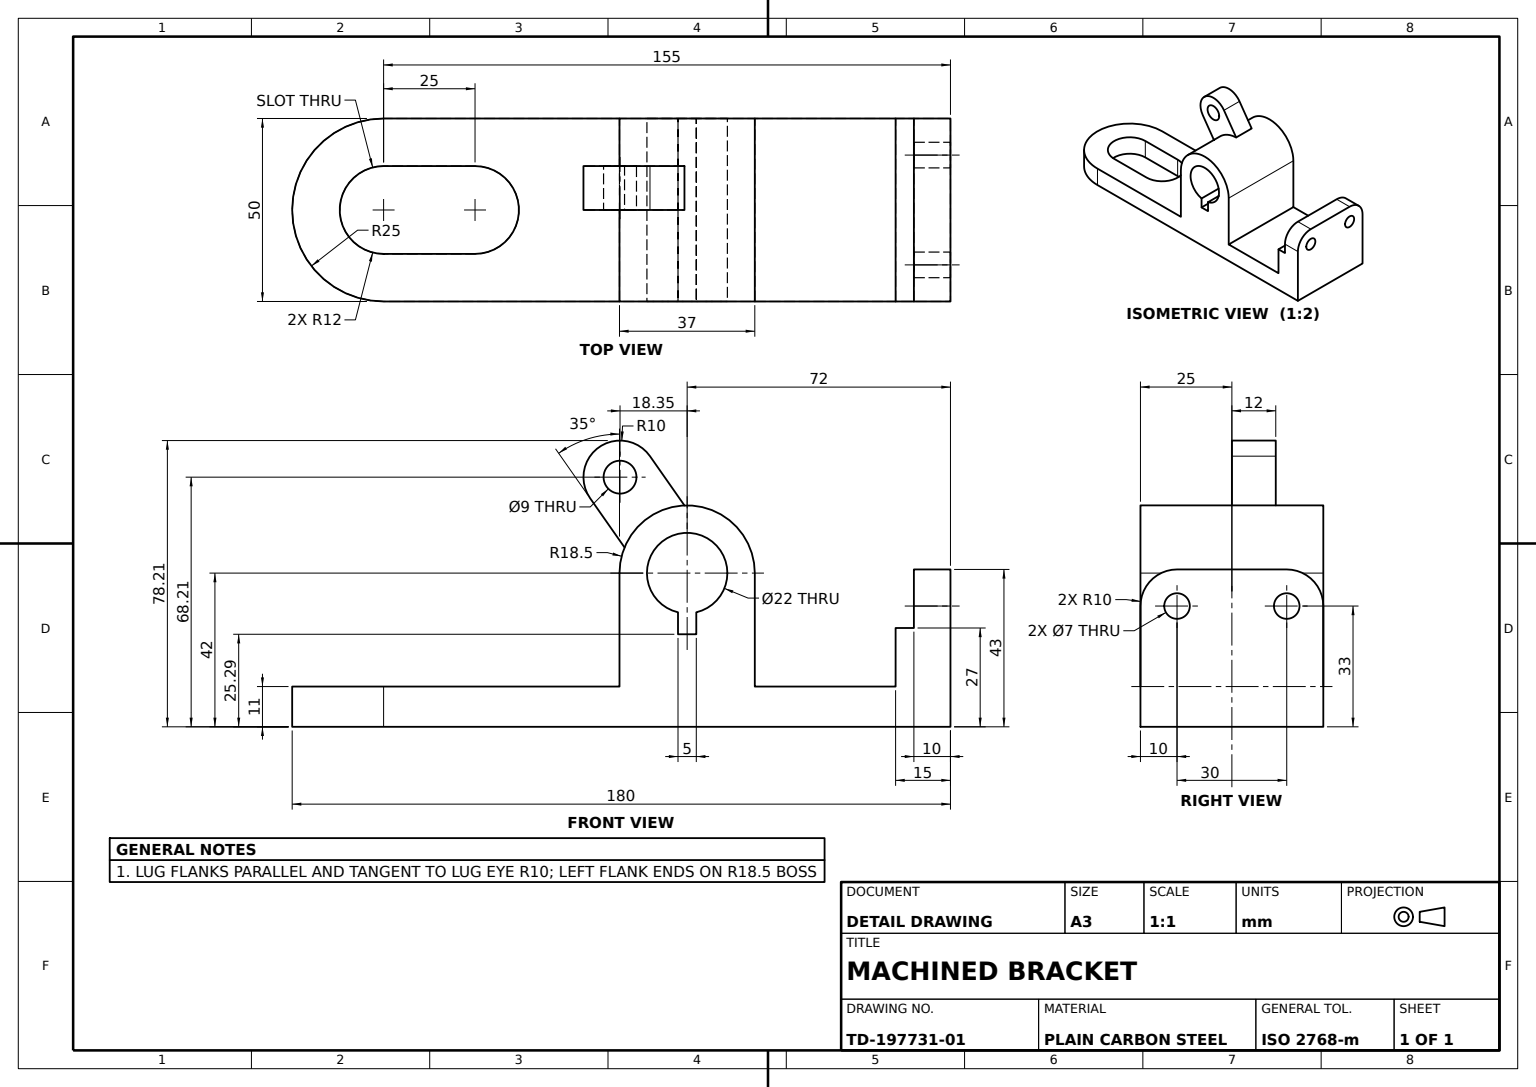
from build123d import *

# Parameters (mm, degrees)
SLOTTED_BASE_PLATE_DEPTH = 11
UPRIGHT_HUB_BODY_DEPTH   = 50
CROSS_START              = 12
CROSS_BOSS_SKETCH_R      = 4.5
CROSS_BOSS_DEPTH         = 12
UPRIGHT_FILLET_R10_R     = 10
CROSS_HOLE_SKETCH_R      = 3.5
CROSS_HOLE_CUT_DEPTH     = 12


with BuildPart() as part:
    # Base Plate Sketch → Slotted Base Plate (new body)
    with BuildSketch(Plane(origin=(0, 0, 0), x_dir=(1, 0, 0), z_dir=(0, 1, 0))):
        with BuildLine():
            Line((0, 25), (-155, 25))
            Line((-155, 25), (-155, -25))
            Line((-155, -25), (0, -25))
            ThreePointArc((0, -25), (25, 0), (0, 25))
        make_face()
        with BuildLine():
            Line((0, -12), (-25, -12))
            ThreePointArc((-25, -12), (-37, 0), (-25, 12))
            Line((-25, 12), (0, 12))
            ThreePointArc((0, 12), (12, 0), (0, -12))
        make_face(mode=Mode.SUBTRACT)
    extrude(amount=SLOTTED_BASE_PLATE_DEPTH)

    # Upright Profile Sketch → Upright Hub Body (add)
    # profile 1 of 2: a face of its own
    with BuildSketch(Plane.XY.offset(25)):
        Polygon((-155, 0), (-155, 43), (-145, 43), (-145, 27), (-140, 27), (-140, 11), align=None)
    # profile 2 of 2: a face of its own
    with BuildSketch(Plane.XY.offset(25)):
        with BuildLine():
            Line((-101.5, 42), (-101.5, 11))
            Line((-101.5, 11), (-64.5, 11))
            Line((-64.5, 11), (-64.5, 42))
            ThreePointArc((-64.5, 42), (-83, 60.5), (-101.5, 42))
        make_face()
        with BuildLine():
            Line((-85.5, 25.287857357), (-80.5, 25.287857357))
            Line((-80.5, 25.287857357), (-80.5, 31.287857357))
            ThreePointArc((-80.5, 31.287857357), (-83, 53), (-85.5, 31.287857357))
            Line((-85.5, 31.287857357), (-85.5, 25.287857357))
        make_face(mode=Mode.SUBTRACT)
    extrude(amount=-UPRIGHT_HUB_BODY_DEPTH)

    # Cross Boss Sketch → Cross Boss (add)
    with BuildSketch(Plane.XY.offset(CROSS_START)):
        with BuildLine():
            Line((-65.881116557, 49.013831311), (-56.454033594, 62.477101054))
            ThreePointArc((-56.454033594, 62.477101054), (-58.909789673, 76.40438586), (-72.83707448, 73.948629781))
            Line((-72.83707448, 73.948629781), (-82.264157443, 60.485360038))
            ThreePointArc((-82.264157443, 60.485360038), (-72.388835928, 57.154312819), (-65.881116557, 49.013831311))
        make_face()
        with Locations((-64.645554037, 68.212865417)):
            Circle(CROSS_BOSS_SKETCH_R, mode=Mode.SUBTRACT)
    extrude(amount=-CROSS_BOSS_DEPTH)

    # Upright Fillet R10
    upright_fillet_r10_edges = [part.edges().sort_by_distance(p)[0] for p in [
        (-150, 43, 25),
        (-150, 43, -25),
    ]]
    fillet(upright_fillet_r10_edges, radius=UPRIGHT_FILLET_R10_R)

    # Cross Hole Sketch → Cross Hole Cut (cut)
    with BuildSketch(Plane.ZY.offset(155)):
        with Locations((15, 33)):
            Circle(CROSS_HOLE_SKETCH_R)
        with Locations((-15, 33)):
            Circle(CROSS_HOLE_SKETCH_R)
    extrude(amount=-CROSS_HOLE_CUT_DEPTH, mode=Mode.SUBTRACT)


solid = part.part
